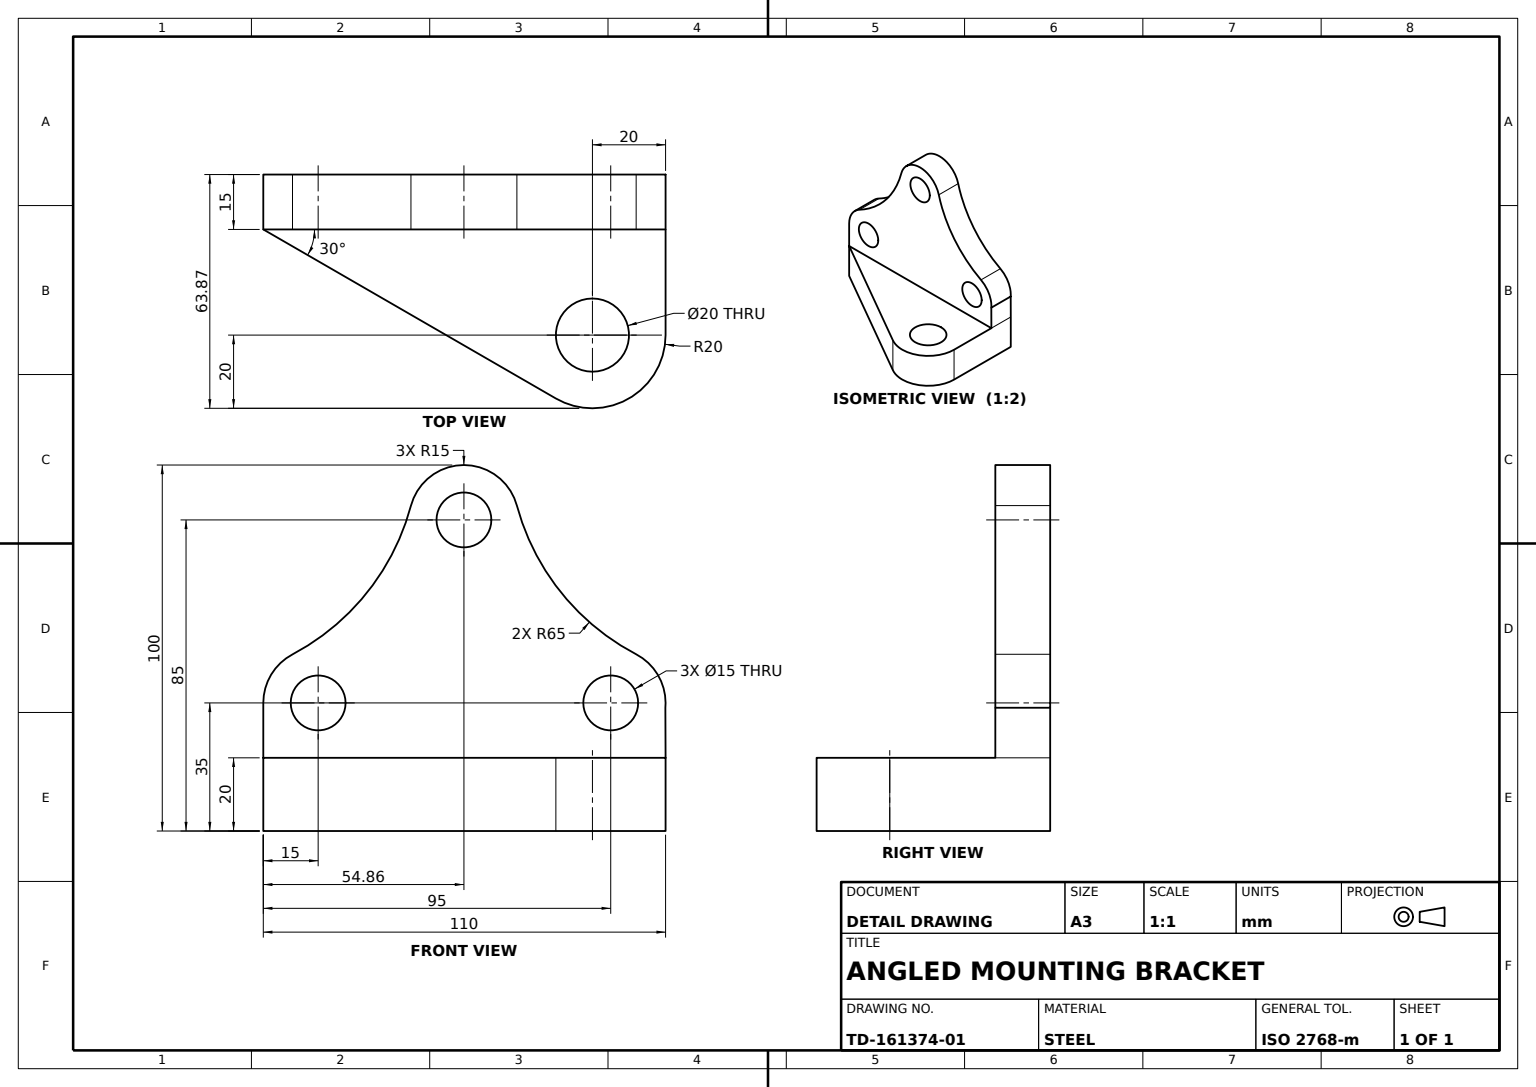
from build123d import *

# Parameters (mm, degrees)
BASE_WEDGE_PROFILE_SKETCH_R     = 10
BASE_WEDGE_BLOCK_DEPTH          = 20
UPRIGHT_FLANGE_PROFILE_SKETCH_R = 7.5
UPRIGHT_FLANGE_PROFILE_SKETCH_W = 110
UPRIGHT_FLANGE_PROFILE_SKETCH_H = 20
UPRIGHT_FLANGE_WITH_HOLES_DEPTH = 15


with BuildPart() as part:
    # Base Wedge Profile Sketch → Base Wedge Block (new body)
    with BuildSketch(Plane(origin=(0, 0, 0), x_dir=(1, 0, 0), z_dir=(0, 1, 0))):
        with BuildLine():
            Line((0, 0), (110, 0))
            Line((110, 0), (110, -28.867513459))
            ThreePointArc((110, -28.867513459), (100, -46.188021535), (80, -46.188021535))
            Line((80, -46.188021535), (0, 0))
        make_face()
        with Locations(Location((90, -28.867513459, 0), (0, 0, 270))):
            Circle(BASE_WEDGE_PROFILE_SKETCH_R, mode=Mode.SUBTRACT)
    extrude(amount=-BASE_WEDGE_BLOCK_DEPTH)

    # Upright Flange Profile Sketch → Upright Flange with Holes (add)
    # profile 1 of 2: a face of its own
    with BuildSketch(Plane(origin=(0, 0, 0), x_dir=(-1, 0, 0), z_dir=(0, 0, -1))):
        with BuildLine():
            ThreePointArc((-40.373259229, 68.883899859), (-28.414925005, 45.194724357), (-7.985616598, 28.258899859))
            ThreePointArc((-7.985616598, 28.258899859), (-2.150569059, 22.739000225), (0, 15))
            Line((0, 15), (0, 0))
            Line((0, 0), (-110, 0))
            Line((-110, 0), (-109.941701745, 13.678807753))
            ThreePointArc((-109.941701745, 13.678807753), (-108.161756455, 22.195009869), (-101.953967939, 28.290685833))
            ThreePointArc((-101.953967939, 28.290685833), (-81.399813181, 45.193056262), (-69.341610571, 68.915685833))
            ThreePointArc((-69.341610571, 68.915685833), (-54.845255035, 79.99999097), (-40.373259229, 68.883899859))
        make_face()
        with Locations((-54.861714008, 65)):
            Circle(UPRIGHT_FLANGE_PROFILE_SKETCH_R, mode=Mode.SUBTRACT)
        with Locations((-15, 15)):
            Circle(UPRIGHT_FLANGE_PROFILE_SKETCH_R, mode=Mode.SUBTRACT)
        with Locations((-95, 15)):
            Circle(UPRIGHT_FLANGE_PROFILE_SKETCH_R, mode=Mode.SUBTRACT)
    # profile 2 of 2: a face of its own
    with BuildSketch(Plane(origin=(0, 0, 0), x_dir=(-1, 0, 0), z_dir=(0, 0, -1))):
        with Locations((-55, -10)):
            Rectangle(UPRIGHT_FLANGE_PROFILE_SKETCH_W, UPRIGHT_FLANGE_PROFILE_SKETCH_H)
    extrude(amount=UPRIGHT_FLANGE_WITH_HOLES_DEPTH)


solid = part.part
